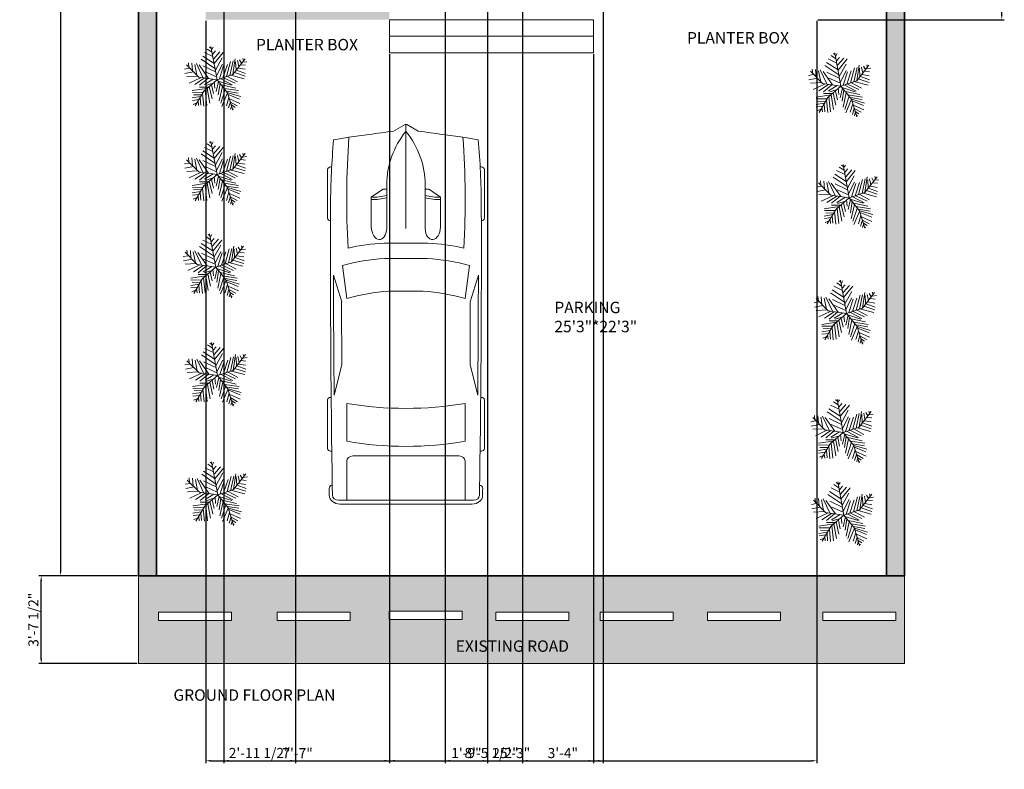
# Model space of a CAD drawing. Units: inches. Extents: x 2130 to 2621, y 981 to 1994.
# Tile 1 of 4: x 2130 to 2618, y 981 to 1353. Entities that reach past the tile are written whole.
import ezdxf

# ---------------------------------------------------------------- set-up
doc = ezdxf.new("R2010")
doc.units = ezdxf.units.IN
for name, color, linetype, lineweight in [('A-ANNO-DIMS', 2, 'Continuous', 18), ('A-ANNO-TEXT', 10, 'Continuous', 18), ('A-AREA-IDEN', 10, 'Continuous', 18), ('A-FLOR-STRS', 7, 'Continuous', 18), ('A-WALL-PATT', 140, 'Continuous', 13), ('C-PARK-VEHI', 8, 'Continuous', 18), ('C-PROP', 7, 'Continuous', 35), ('C-PROP-PATT', 140, 'Continuous', 13), ('C-ROAD-PATT', 252, 'Continuous', 13), ('ROAD', 18, 'Continuous', 18), ('TREE', 112, 'Continuous', 18)]:
    doc.layers.add(name, color=color, linetype=linetype, lineweight=lineweight)
doc.styles.get("Standard").update_dxf_attribs({"font": 'arial.ttf'})
doc.dimstyles.new('ISO-25', dxfattribs={"dimtxt": 5, "dimasz": 2.5, "dimexe": 1.25, "dimexo": 0.625, "dimtad": 1, "dimdec": 0, "dimlunit": 4, "dimtxsty": 'Standard', "dimcen": 2.5, "dimadec": 0, "dimazin": 0, "dimtfac": 1, "dimtdec": 0, "dimtmove": 0, "dimatfit": 3, "dimfxl": 1, "dimarcsym": 0})

# ---------------------------------------------------------------- blocks, each defined once
blk = doc.blocks.new('*U6')
for p, q in [((21.1, 37.41), (21.1, 36.83)), ((46.55, 38.89), (22.35, 38.89)), ((47.8, 37.39), (47.8, 37.41)), ((87.99, 31.87), (74.76, 35.92)), ((134.31, 35.6), (119.29, 31.78)), ((135.45, 37.07), (135.45, 37.41)), ((136.7, 38.89), (160.9, 38.89)), ((162.15, 37.41), (162.15, 36.77)), ((70.03, 31.54), (86.41, 29.35)), ((138.42, 29.35), (157.25, 29.35)), ((186.47, 29.35), (167.01, 29.35)), ((186.47, -33.5), (186.47, 33.5)), ((188.4, -32.76), (188.4, 32.76)), ((164.52, 26.39), (164.52, -26.39)), ((32.27, 11.63), (36.13, 17.17)), ((36.13, 17.17), (50.94, 17.17)), ((32.12, 9.51), (32.12, 11.15)), ((58.92, -10.77), (58.92, 10.77)), ((66.55, -10.53), (66.55, 10.53)), ((186.47, -10.53), (186.47, 10.53)), ((3.27, 6.13), (0.1, 0.41)), ((29.77, 9.51), (51.68, 9.51)), ((82.74, 8.5), (82.74, -8.5)), ((0, 0), (51.68, 0)), ((0.1, -0.41), (3.27, -6.13)), ((29.77, -9.51), (51.68, -9.51)), ((32.12, -9.51), (32.12, -11.15)), ((32.27, -11.63), (36.13, -17.17)), ((36.13, -17.17), (50.94, -17.17)), ((86.41, -29.35), (70.03, -31.54)), ((87.99, -31.87), (74.76, -35.92)), ((134.31, -35.6), (119.29, -31.78)), ((157.25, -29.35), (138.42, -29.35)), ((167.01, -29.35), (186.47, -29.35)), ((21.1, -37.41), (21.1, -36.83)), ((46.55, -38.89), (22.35, -38.89)), ((47.8, -37.39), (47.8, -37.41)), ((135.45, -37.07), (135.45, -37.41)), ((136.7, -38.89), (160.9, -38.89)), ((162.15, -37.41), (162.15, -36.77))]:
    blk.add_line(p, q)
for centre, major_axis, ratio, start_param, end_param in [((266.03, -27.52), (0, 313.31), 0.842304, 1.367076, 1.39176), ((41.19, -490.86), (0, 528.23), 0.842304, 0.00281, 0.075598), ((22.35, 37.41), (0, -1.48), 0.842304, 3.141593, 4.712389), ((64.48, -10555.62), (0, 10593.03), 0.842304, -0.013397, 0.002797), ((46.55, 37.41), (0, 1.48), 0.842304, -1.570796, 0), ((64.48, -10555.62), (0, -10591.55), 0.842304, 3.133765, 3.140441), ((136.7, 37.41), (0, -1.48), 0.842304, 3.141593, 4.712389), ((160.9, 37.41), (0, 1.48), 0.842304, -1.570796, 0), ((180.63, 35.84), (0, 2.22), 0.842304, -0.013017, 1.249894), ((64.48, -10556.36), (0, 10595.31), 0.842304, -0.013397, -0.013017), ((183.98, 33.5), (0, -2.96), 0.842304, 1.570796, 3.128196), ((183.98, 32.76), (0, -5.25), 0.842304, 1.570796, 3.128196), ((37.47, -593.96), (0, -623.33), 0.842304, 3.096046, 3.200911), ((135.29, 5.39), (0, 81.77), 0.842304, 1.245306, 1.50788), ((149.6, 2.8), (0, -79.58), 0.842304, 4.372215, 4.640744), ((95.79, -3666.35), (0, -3698.24), 0.842304, 3.134049, 3.144098), ((17.08, 0), (0, 147.02), 0.842304, 4.511394, 4.913384), ((35.91, 0), (0, 147.02), 0.842304, 4.511394, 4.913384), ((167.01, 26.39), (0, 2.96), 0.842304, 0, 1.570796), ((259.18, -27.52), (0, -305.3), 0.842304, 4.528606, 4.561838), ((134.4, 5.39), (0, -89.78), 0.842304, 4.449482, 4.652344), ((-204.49, 52.4), (0, -250.96), 0.842304, 1.385369, 1.434372), ((13.04, 17.01), (0, 27.42), 0.842304, 4.435146, 4.718221), ((14.2, 17.01), (0, 27.42), 0.842304, 4.435146, 4.718221), ((50.79, 13.34), (6.34, -0.36), 0.603834, -1.395552, 1.581315), ((32.75, 11.15), (0, 0.74), 0.842304, 0.879714, 1.570796), ((29.77, -46.66), (0, 56.17), 0.842304, 0, 0.590319), ((0.62, 0), (0, -0.74), 0.842304, 4.131459, 5.293319), ((29.77, 46.66), (0, 56.17), 0.842304, 2.551274, 3.141593), ((-204.49, -52.4), (0, 250.96), 0.842304, -1.434372, -1.385369), ((13.04, -17.01), (0, -27.42), 0.842304, 1.564964, 1.848039), ((14.2, -17.01), (0, -27.42), 0.842304, 1.564964, 1.848039), ((149.6, -2.8), (0, -79.58), 0.842304, -1.499151, -1.230623), ((32.75, -11.15), (0, -0.74), 0.842304, 4.712389, 5.403472), ((134.4, -5.39), (0, -89.78), 0.842304, -1.510751, -1.307889), ((135.29, -5.39), (0, -81.77), 0.842304, -1.50788, -1.245306), ((259.18, 27.52), (0, 305.3), 0.842304, 1.721348, 1.754579), ((266.03, 27.52), (0, 313.31), 0.842304, 1.749832, 1.774517), ((37.47, 593.96), (0, -623.33), 0.842304, -0.059319, 0.045547), ((167.01, -26.39), (0, -2.96), 0.842304, 4.712389, 6.283185), ((95.79, 3666.35), (0, -3698.24), 0.842304, -0.002505, 0.007544), ((183.98, -33.5), (0, 2.96), 0.842304, 3.15499, 4.712389), ((183.98, -32.76), (0, -5.25), 0.842304, 0.013397, 1.570796), ((41.19, 490.86), (0, -528.23), 0.842304, -0.075598, -0.00281), ((22.35, -37.41), (0, 1.48), 0.842304, 1.570796, 3.141593), ((64.48, 10555.62), (0, 10593.03), 0.842304, 3.138796, 3.15499), ((46.55, -37.41), (0, -1.48), 0.842304, 0, 1.570796), ((64.48, 10555.62), (0, -10591.55), 0.842304, 0.001152, 0.007828), ((136.7, -37.41), (0, -1.48), 0.842304, -1.570796, 0), ((160.9, -37.41), (0, 1.48), 0.842304, 3.141593, 4.712389), ((180.63, -35.84), (0, -2.22), 0.842304, -1.249894, 0.013017), ((64.48, 10556.36), (0, 10595.31), 0.842304, 3.15461, 3.15499)]:
    blk.add_ellipse(centre, major_axis=major_axis, ratio=ratio, start_param=start_param, end_param=end_param)
at = {"extrusion": (0, 0, -1)}
blk.add_ellipse((50.79, -13.34), major_axis=(6.34, 0.36), ratio=0.603834, start_param=-1.395552, end_param=1.581315, dxfattribs=at)
blk = doc.blocks.new('*D10')
at = {"layer": 'A-ANNO-DIMS', "color": 0, "lineweight": -2, "transparency": 16777216}
for p, q in [((2188.13, 1935.02), (2148.94, 1935.02)), ((2150.19, 1932.52), (2150.19, 1079.91)), ((2188.13, 1077.41), (2148.94, 1077.41))]:
    blk.add_line(p, q, dxfattribs=at)
at = {"layer": 'A-ANNO-DIMS', "color": 0, "transparency": 16777216}
for points in [[(2149.77, 1932.52), (2150.61, 1932.52), (2150.19, 1935.02)], [(2149.77, 1079.91), (2150.61, 1079.91), (2150.19, 1077.41)]]:
    blk.add_solid(points, dxfattribs=at)
at = {"layer": 'Defpoints', "color": 0, "transparency": 16777216}
for p in [(2188.76, 1935.02), (2150.19, 1077.41), (2188.76, 1077.41)]:
    blk.add_point(p, dxfattribs=at)
at = {"layer": 'A-ANNO-DIMS', "color": 0, "transparency": 16777216, "insert": (2147.01, 1506.21), "char_height": 5, "attachment_point": 5, "rotation": 90}
blk.add_mtext('71\'-6"', dxfattribs=at)
blk = doc.blocks.new('*U8')
for p, q in [((-8.737, 47.138), (-17.069, 52.711)), ((-10.186, 53.64), (-13.084, 55.962)), ((0, 0), (-10.5, 57)), ((-9.099, 51.782), (-6.563, 55.962)), ((-3.665, 19.273), (-27.574, 35.527)), ((-5.114, 28.097), (-24.676, 40.636)), ((-7.288, 39.707), (-21.778, 46.673)), ((-7.65, 43.423), (-2.578, 49.46)), ((-5.839, 35.992), (4.667, 48.067)), ((-5.114, 27.632), (10.463, 46.673)), ((-2.941, 16.486), (8.652, 37.85)), ((27, 9), (48, 36)), ((27.127, 9.056), (31.112, 35.992)), ((38.719, 34.134), (41.979, 28.561)), ((44.153, 36.456), (45.239, 32.741)), ((-47.498, 19.737), (-55.83, 18.344)), ((-31.5, 4.5), (-52.5, 25.5)), ((-48.585, 21.131), (-49.309, 29.026)), ((-43.513, 28.561), (-42.427, 15.558)), ((-38.442, 26.239), (-34.819, 7.663)), ((-35.544, 28.097), (-24.314, 3.947)), ((-14.533, 2.09), (-30.834, 25.31)), ((-24.314, 23.917), (-2.941, 13.7)), ((-1.129, 6.734), (9.014, 26.704)), ((3.942, 1.625), (11.187, 24.381)), ((10.101, 3.483), (17.708, 26.239)), ((16.259, 5.805), (23.142, 31.348)), ((22.055, 7.198), (27.489, 32.277)), ((31.836, 30.883), (32.561, 16.486)), ((35.096, 32.741), (37.27, 22.524)), ((36.183, 19.737), (48.137, 17.88)), ((40.53, 25.775), (48.862, 24.846)), ((43.791, 29.954), (51.036, 30.883)), ((-40.615, 13.7), (-55.105, 10.913)), ((-33.37, 6.269), (-52.207, 5.34)), ((-28.299, 3.483), (-47.86, -5.805)), ((-21.416, 3.018), (-38.079, -8.128)), ((0, 0), (-31.5, 4.5)), ((-15.982, 2.09), (-30.11, -9.521)), ((0, 0), (-22.5, -19.5)), ((-6.563, 1.161), (-21.416, -8.128)), ((-20.691, 13.7), (-1.129, 4.876)), ((0, 0), (27, 9)), ((0, 0), (18, -22.5)), ((6.478, 1.625), (26.04, -8.592)), ((11.187, 3.483), (30.749, -5.805)), ((18.07, 5.805), (35.096, -3.483)), ((24.229, 7.663), (46.688, 1.625)), ((29.662, 12.307), (48.137, 6.269)), ((33.285, 16.486), (48.862, 10.913)), ((-17.431, -15.094), (-42.789, -18.809)), ((-15.257, -12.772), (-30.11, -12.772)), ((-6.563, -5.805), (-19.967, -9.985)), ((-17.069, -15.094), (-12.721, -40.172)), ((-13.446, -11.378), (-8.737, -32.741)), ((-9.461, -8.592), (-6.201, -23.453)), ((-4.752, -3.483), (-3.665, -14.629)), ((2.493, -3.019), (-1.491, -20.202)), ((1.769, -2.555), (24.229, -9.521)), ((5.029, -6.27), (2.131, -25.775)), ((9.014, -11.378), (3.58, -35.992)), ((7.565, -9.056), (32.198, -14.629)), ((12.274, -15.094), (36.907, -18.809)), ((-28.299, -29.026), (-42.789, -31.348)), ((-24.314, -21.596), (-42.427, -22.06)), ((-26.849, -26.24), (-40.253, -25.775)), ((-22.5, -19.5), (-37.5, -45)), ((-29.023, -30.884), (-27.936, -43.887)), ((-25.038, -23.918), (-22.865, -45.281)), ((-20.691, -18.345), (-17.793, -44.352)), ((14.085, -16.951), (6.478, -40.172)), ((18.07, -22.524), (8.289, -45.745)), ((20.244, -30.419), (15.897, -44.816)), ((16.259, -19.738), (36.183, -22.989)), ((18, -22.5), (27, -52.5)), ((18.433, -22.524), (40.53, -29.026)), ((19.157, -25.311), (38.719, -33.206)), ((21.331, -32.741), (39.081, -40.636)), ((-30.834, -34.135), (-42.427, -35.528)), ((-34.457, -39.708), (-40.978, -42.494)), ((-32.646, -36.921), (-31.921, -44.352)), ((22.78, -37.85), (19.519, -48.532)), ((22.78, -38.314), (34.372, -44.816)), ((24.591, -45.745), (23.142, -50.854)), ((24.591, -43.423), (30.749, -47.603)), ((26.764, -49.925), (28.213, -50.854))]:
    blk.add_line(p, q)
blk = doc.blocks.new('*D23')
at = {"layer": 'A-ANNO-DIMS', "color": 0, "lineweight": -2, "transparency": 16777216}
for p, q in [((2222.16, 1352.79), (2222.16, 984.42)), ((2525.16, 1352.79), (2525.16, 984.42)), ((2224.66, 985.67), (2522.66, 985.67))]:
    blk.add_line(p, q, dxfattribs=at)
at = {"layer": 'A-ANNO-DIMS', "color": 0, "transparency": 16777216}
for points in [[(2224.66, 986.08), (2224.66, 985.25), (2222.16, 985.67)], [(2522.66, 986.08), (2522.66, 985.25), (2525.16, 985.67)]]:
    blk.add_solid(points, dxfattribs=at)
at = {"layer": 'Defpoints', "color": 0, "transparency": 16777216}
for p in [(2222.16, 1353.41), (2525.16, 1353.41), (2525.16, 985.67)]:
    blk.add_point(p, dxfattribs=at)
at = {"layer": 'A-ANNO-DIMS', "color": 0, "transparency": 16777216, "insert": (2373.66, 988.85), "char_height": 5, "attachment_point": 5}
blk.add_mtext('25\'-3"', dxfattribs=at)
blk = doc.blocks.new('*D24')
at = {"layer": 'A-ANNO-DIMS', "color": 0, "lineweight": -2, "transparency": 16777216}
for p, q in [((2525.79, 1890.41), (2618.19, 1890.41)), ((2616.94, 1355.91), (2616.94, 1887.91)), ((2525.79, 1353.41), (2618.19, 1353.41))]:
    blk.add_line(p, q, dxfattribs=at)
at = {"layer": 'A-ANNO-DIMS', "color": 0, "transparency": 16777216}
for points in [[(2616.52, 1887.91), (2617.35, 1887.91), (2616.94, 1890.41)], [(2616.52, 1355.91), (2617.35, 1355.91), (2616.94, 1353.41)]]:
    blk.add_solid(points, dxfattribs=at)
at = {"layer": 'Defpoints', "color": 0, "transparency": 16777216}
for p in [(2525.16, 1890.41), (2616.94, 1890.41), (2525.16, 1353.41)]:
    blk.add_point(p, dxfattribs=at)
at = {"layer": 'A-ANNO-DIMS', "color": 0, "transparency": 16777216, "insert": (2613.76, 1621.91), "char_height": 5, "attachment_point": 5, "rotation": 90}
blk.add_mtext('44\'-9"', dxfattribs=at)
blk = doc.blocks.new('*D27')
at = {"layer": 'A-ANNO-DIMS', "color": 0, "lineweight": -2, "transparency": 16777216}
for p, q in [((2188.13, 1077.41), (2139.33, 1077.41)), ((2140.58, 1036.35), (2140.58, 1074.91)), ((2188.13, 1033.85), (2139.33, 1033.85))]:
    blk.add_line(p, q, dxfattribs=at)
at = {"layer": 'A-ANNO-DIMS', "color": 0, "transparency": 16777216}
for points in [[(2140.16, 1074.91), (2140.99, 1074.91), (2140.58, 1077.41)], [(2140.16, 1036.35), (2140.99, 1036.35), (2140.58, 1033.85)]]:
    blk.add_solid(points, dxfattribs=at)
at = {"layer": 'Defpoints', "color": 0, "transparency": 16777216}
for p in [(2140.58, 1077.41), (2188.76, 1077.41), (2188.76, 1033.85)]:
    blk.add_point(p, dxfattribs=at)
at = {"layer": 'A-ANNO-DIMS', "color": 0, "transparency": 16777216, "insert": (2137.36, 1055.63), "char_height": 5, "attachment_point": 5, "rotation": 90}
blk.add_mtext('3\'-7 1/2"', dxfattribs=at)
blk = doc.blocks.new('*D30')
at = {"layer": 'A-ANNO-DIMS', "color": 0, "lineweight": -2, "transparency": 16777216}
for p, q in [((2313.28, 1336.32), (2313.28, 984.42)), ((2414.54, 1336.32), (2414.54, 984.42)), ((2315.78, 985.67), (2412.04, 985.67))]:
    blk.add_line(p, q, dxfattribs=at)
at = {"layer": 'A-ANNO-DIMS', "color": 0, "transparency": 16777216}
for points in [[(2315.78, 986.08), (2315.78, 985.25), (2313.28, 985.67)], [(2412.04, 986.08), (2412.04, 985.25), (2414.54, 985.67)]]:
    blk.add_solid(points, dxfattribs=at)
at = {"layer": 'Defpoints', "color": 0, "transparency": 16777216}
for p in [(2313.28, 1336.95), (2414.54, 1336.95), (2414.54, 985.67)]:
    blk.add_point(p, dxfattribs=at)
at = {"layer": 'A-ANNO-DIMS', "color": 0, "transparency": 16777216, "insert": (2363.91, 988.88), "char_height": 5, "attachment_point": 5}
blk.add_mtext('8\'-5 1/2"', dxfattribs=at)
blk = doc.blocks.new('*D31')
at = {"layer": 'A-ANNO-DIMS', "color": 0, "lineweight": -2, "transparency": 16777216}
for p, q in [((2222.16, 1352.79), (2222.16, 984.42)), ((2313.28, 1336.32), (2313.28, 984.42)), ((2224.66, 985.67), (2310.78, 985.67))]:
    blk.add_line(p, q, dxfattribs=at)
at = {"layer": 'A-ANNO-DIMS', "color": 0, "transparency": 16777216}
for points in [[(2224.66, 986.08), (2224.66, 985.25), (2222.16, 985.67)], [(2310.78, 986.08), (2310.78, 985.25), (2313.28, 985.67)]]:
    blk.add_solid(points, dxfattribs=at)
at = {"layer": 'Defpoints', "color": 0, "transparency": 16777216}
for p in [(2222.16, 1353.41), (2313.28, 1336.95), (2313.28, 985.67)]:
    blk.add_point(p, dxfattribs=at)
at = {"layer": 'A-ANNO-DIMS', "color": 0, "transparency": 16777216, "insert": (2267.72, 988.79), "char_height": 5, "attachment_point": 5}
blk.add_mtext('7\'-7"', dxfattribs=at)
blk = doc.blocks.new('*D33')
at = {"layer": 'A-ANNO-DIMS', "color": 0, "lineweight": -2, "transparency": 16777216}
for p, q in [((2231.16, 1510.29), (2231.16, 984.42)), ((2266.66, 1510.29), (2266.66, 984.42)), ((2233.66, 985.67), (2264.16, 985.67))]:
    blk.add_line(p, q, dxfattribs=at)
at = {"layer": 'A-ANNO-DIMS', "color": 0, "transparency": 16777216}
for points in [[(2233.66, 986.08), (2233.66, 985.25), (2231.16, 985.67)], [(2264.16, 986.08), (2264.16, 985.25), (2266.66, 985.67)]]:
    blk.add_solid(points, dxfattribs=at)
at = {"layer": 'Defpoints', "color": 0, "transparency": 16777216}
for p in [(2231.16, 1510.91), (2266.66, 1510.91), (2266.66, 985.67)]:
    blk.add_point(p, dxfattribs=at)
at = {"layer": 'A-ANNO-DIMS', "color": 0, "transparency": 16777216, "insert": (2248.91, 988.88), "char_height": 5, "attachment_point": 5}
blk.add_mtext('2\'-11 1/2"', dxfattribs=at)
blk = doc.blocks.new('*D36')
at = {"layer": 'A-ANNO-DIMS', "color": 0, "lineweight": -2, "transparency": 16777216}
for p, q in [((2379.27, 1730.79), (2379.27, 984.42)), ((2419.27, 1730.79), (2419.27, 984.42)), ((2381.77, 985.67), (2416.77, 985.67))]:
    blk.add_line(p, q, dxfattribs=at)
at = {"layer": 'A-ANNO-DIMS', "color": 0, "transparency": 16777216}
for points in [[(2381.77, 986.08), (2381.77, 985.25), (2379.27, 985.67)], [(2416.77, 986.08), (2416.77, 985.25), (2419.27, 985.67)]]:
    blk.add_solid(points, dxfattribs=at)
at = {"layer": 'Defpoints', "color": 0, "transparency": 16777216}
for p in [(2379.27, 1731.41), (2419.27, 1731.41), (2419.27, 985.67)]:
    blk.add_point(p, dxfattribs=at)
at = {"layer": 'A-ANNO-DIMS', "color": 0, "transparency": 16777216, "insert": (2399.27, 988.85), "char_height": 5, "attachment_point": 5}
blk.add_mtext('3\'-4"', dxfattribs=at)
blk = doc.blocks.new('*D45')
at = {"layer": 'A-ANNO-DIMS', "color": 0, "lineweight": -2, "transparency": 16777216}
for p, q in [((2340.91, 1828.29), (2340.91, 984.42)), ((2361.98, 1828.29), (2361.98, 984.42)), ((2343.41, 985.67), (2359.48, 985.67))]:
    blk.add_line(p, q, dxfattribs=at)
at = {"layer": 'A-ANNO-DIMS', "color": 0, "transparency": 16777216}
for points in [[(2343.41, 986.08), (2343.41, 985.25), (2340.91, 985.67)], [(2359.48, 986.08), (2359.48, 985.25), (2361.98, 985.67)]]:
    blk.add_solid(points, dxfattribs=at)
at = {"layer": 'Defpoints', "color": 0, "transparency": 16777216}
for p in [(2340.91, 1828.91), (2361.98, 1828.91), (2361.98, 985.67)]:
    blk.add_point(p, dxfattribs=at)
at = {"layer": 'A-ANNO-DIMS', "color": 0, "transparency": 16777216, "insert": (2351.44, 988.84), "char_height": 5, "attachment_point": 5}
blk.add_mtext('1\'-9"', dxfattribs=at)

msp = doc.modelspace()

# ---------------------------------------------------------------- hatches: boundary and pattern name
at = {"layer": 'A-WALL-PATT'}
h = msp.add_hatch(color=256, dxfattribs=at)
h.dxf.hatch_style = 1
h.paths.add_polyline_path([(2231.16, 1595.8), (2222.16, 1595.8), (2222.16, 1571.6), (2225.81, 1571.6), (2231.16, 1571.6)])
h.paths.add_polyline_path([(2313.28, 1362.41), (2237.26, 1362.41), (2231.16, 1362.41), (2231.16, 1404.41), (2231.16, 1474.85), (2231.16, 1547.86, -0.05547), (2225.81, 1547.27), (2222.16, 1547.27), (2222.16, 1425.41), (2222.16, 1353.41), (2313.28, 1353.41)])
h.paths.add_polyline_path([(2393.01, 1195.09), (2434.46, 1195.09), (2434.46, 1216.28), (2393.01, 1216.28)], flags=9)
h.paths.add_polyline_path([(2245.08, 1335), (2303.47, 1335), (2303.47, 1346.7), (2245.08, 1346.7)], flags=9)
h.paths.add_polyline_path([(2458.81, 1338.38), (2517.21, 1338.38), (2517.21, 1350.09), (2458.81, 1350.09)], flags=9)
h.paths.add_polyline_path([(2232.7, 1530.42), (2263.31, 1530.42), (2263.31, 1551.62), (2232.7, 1551.62)], flags=9)
h.paths.add_polyline_path([(2332.94, 1458.61), (2399.05, 1458.61), (2399.05, 1489.37), (2332.94, 1489.37)], flags=9)
h.paths.add_polyline_path([(2475.66, 1607.66), (2507.9, 1607.66), (2507.9, 1628.85), (2475.66, 1628.85)], flags=9)
h.paths.add_polyline_path([(2486.7, 1688.97), (2517.32, 1688.97), (2517.32, 1710.17), (2486.7, 1710.17)], flags=9)
h.paths.add_polyline_path([(2333.88, 1649.81), (2375.07, 1649.81), (2375.07, 1671), (2333.88, 1671)], flags=9)
h.paths.add_polyline_path([(2441.42, 1774.34), (2500.24, 1774.34), (2500.24, 1795.53), (2441.42, 1795.53)], flags=9)
h.paths.add_polyline_path([(2332.74, 1857.16), (2363.5, 1857.16), (2363.5, 1878.35), (2332.74, 1878.35)], flags=9)
h.paths.add_polyline_path([(2244.84, 1853.21), (2275.6, 1853.21), (2275.6, 1874.4), (2244.84, 1874.4)], flags=9)
at = {"layer": 'C-PROP-PATT'}
h = msp.add_hatch(color=256, dxfattribs=at)
h.dxf.hatch_style = 1
h.paths.add_polyline_path([(2559.76, 1935.02), (2197.76, 1935.02), (2197.76, 1926.02), (2559.76, 1926.02)])
h.paths.add_polyline_path([(2197.76, 1935.02), (2188.76, 1935.02), (2188.76, 1077.41), (2197.76, 1077.41)])
h.paths.add_polyline_path([(2568.76, 1926.02), (2559.76, 1926.02), (2559.76, 1077.41), (2568.76, 1077.41)])
h.paths.add_polyline_path([(2568.76, 1935.02), (2559.76, 1935.02), (2559.76, 1926.02), (2568.76, 1926.02)])
at = {"layer": 'C-ROAD-PATT'}
h = msp.add_hatch(color=256, dxfattribs=at)
h.dxf.hatch_style = 1
h.paths.add_polyline_path([(2568.76, 1077.41), (2559.76, 1077.41), (2188.76, 1077.41), (2188.76, 1033.85), (2568.76, 1033.85)])
h.paths.add_polyline_path([(2349.31, 1059.97), (2349.31, 1055.82), (2313.18, 1055.82), (2313.18, 1059.97)], flags=16)
h.paths.add_polyline_path([(2366.11, 1059.44), (2402.25, 1059.44), (2402.25, 1055.28), (2366.11, 1055.28)], flags=16)
h.paths.add_polyline_path([(2417.78, 1059.44), (2453.92, 1059.44), (2453.92, 1055.28), (2417.78, 1055.28)], flags=16)
h.paths.add_polyline_path([(2293.74, 1059.44), (2293.74, 1055.28), (2257.61, 1055.28), (2257.61, 1059.44)], flags=16)
h.paths.add_polyline_path([(2471.02, 1059.44), (2507.15, 1059.44), (2507.15, 1055.28), (2471.02, 1055.28)], flags=16)
h.paths.add_polyline_path([(2234.9, 1059.44), (2234.9, 1055.28), (2198.77, 1055.28), (2198.77, 1059.44)], flags=16)
h.paths.add_polyline_path([(2528.27, 1059.44), (2564.4, 1059.44), (2564.4, 1055.28), (2528.27, 1055.28)], flags=16)
h.paths.add_polyline_path([(2344.06, 1036.51), (2409.07, 1036.51), (2409.07, 1048.22), (2344.06, 1048.22)], flags=24)

# ---------------------------------------------------------------- linework, layer by layer
at = {"layer": 'A-FLOR-STRS'}
for points in [[(2313.28, 1353.41), (2414.44, 1353.41), (2414.44, 1345.18), (2313.28, 1345.18)], [(2313.28, 1345.18), (2414.54, 1345.18), (2414.54, 1336.95), (2313.28, 1336.95)]]:
    msp.add_lwpolyline(points, close=True, dxfattribs=at)
at = {"layer": 'C-PROP'}
for p, q in [((2188.76, 1935.02), (2188.76, 1077.41)), ((2568.76, 1935.02), (2568.76, 1077.41)), ((2197.76, 1926.02), (2197.76, 1086.41)), ((2559.76, 1926.02), (2559.76, 1086.41)), ((2197.76, 1086.41), (2197.76, 1077.41)), ((2559.76, 1086.41), (2559.76, 1077.41)), ((2568.76, 1077.41), (2188.76, 1077.41))]:
    msp.add_line(p, q, dxfattribs=at)
for points in [[(2188.76, 1935.02), (2197.76, 1935.02), (2197.76, 1077.41), (2188.76, 1077.41)], [(2559.76, 1077.41), (2568.76, 1077.41), (2568.76, 1935.02), (2559.76, 1935.02)]]:
    msp.add_lwpolyline(points, close=True, dxfattribs=at)
at = {"layer": 'ROAD'}
for p, q in [((2188.76, 1077.41), (2188.76, 1033.85)), ((2568.76, 1033.85), (2568.76, 1077.41)), ((2188.76, 1033.85), (2568.76, 1033.85))]:
    msp.add_line(p, q, dxfattribs=at)
for points in [[(2313.18, 1059.97), (2349.31, 1059.97), (2349.31, 1055.82), (2313.18, 1055.82)], [(2198.77, 1059.44), (2234.9, 1059.44), (2234.9, 1055.28), (2198.77, 1055.28)], [(2257.61, 1059.44), (2293.74, 1059.44), (2293.74, 1055.28), (2257.61, 1055.28)], [(2366.11, 1059.44), (2402.25, 1059.44), (2402.25, 1055.28), (2366.11, 1055.28)], [(2417.78, 1059.44), (2453.92, 1059.44), (2453.92, 1055.28), (2417.78, 1055.28)], [(2471.02, 1059.44), (2507.15, 1059.44), (2507.15, 1055.28), (2471.02, 1055.28)], [(2528.27, 1059.44), (2564.4, 1059.44), (2564.4, 1055.28), (2528.27, 1055.28)]]:
    msp.add_lwpolyline(points, close=True, dxfattribs=at)

# ---------------------------------------------------------------- block references
at = {"layer": 'C-PARK-VEHI', "rotation": 270}
msp.add_blockref('*U6', (2321.45, 1301.43), dxfattribs=at)
at = {"layer": 'TREE', "xscale": 0.2888583255647464, "yscale": 0.2888583255647464, "zscale": 0.2888583255647464}
for p in [(2227.8, 1323.62), (2537.2, 1320.43), (2227.8, 1276.57), (2541.25, 1265.04), (2227.1, 1230.6), (2540, 1207.62), (2228.01, 1176.8), (2538.33, 1148.63), (2228.14, 1117.6), (2538.65, 1107.56)]:
    msp.add_blockref('*U8', p, dxfattribs=at)

# ---------------------------------------------------------------- texts
at = {"layer": 'A-ANNO-TEXT', "char_height": 5.6797, "attachment_point": 1}
for s, width, insert in [('PLANTER BOX', 57.6358, (2247.11, 1343.88)), ('PLANTER BOX', 57.6358, (2460.84, 1347.27)), ('EXISTING ROAD', 79.6446, (2346.11, 1045.4)), ('GROUND FLOOR PLAN', 98.7305, (2206.15, 1021.11))]:
    msp.add_mtext_dynamic_manual_height_columns(s, width=width, gutter_width=28.4, heights=[0], dxfattribs=dict(at, insert=insert))
at = {"layer": 'A-AREA-IDEN', "insert": (2395.04, 1213.46), "char_height": 5.6797, "attachment_point": 1}
msp.add_mtext_dynamic_manual_height_columns('PARKING\\P25\'3"*22\'3"', width=57.6358, gutter_width=28.4, heights=[0], dxfattribs=at)

# ---------------------------------------------------------------- dimensions: what is measured, and where the dimension line sits
at = {"layer": 'A-ANNO-DIMS'}
for base, p1, p2, override, picture, middle in [((2150.19, 1077.41), (2188.76, 1935.02), (2188.76, 1077.41), {"dimclrd": 0, "dimclre": 0, "dimclrt": 0}, '*D10', (2147.01, 1506.21)), ((2616.94, 1890.41), (2525.16, 1353.41), (2525.16, 1890.41), {"dimdec": 1, "dimlfac": 1, "dimrnd": 0, "dimzin": 1, "dimdsep": 46, "dimlunit": 4, "dimfrac": 2}, '*D24', (2613.76, 1621.91)), ((2140.58, 1077.41), (2188.76, 1033.85), (2188.76, 1077.41), {"dimdec": 1, "dimlfac": 1, "dimrnd": 0, "dimzin": 1, "dimdsep": 46, "dimlunit": 4, "dimfrac": 2}, '*D27', (2137.36, 1055.63))]:
    dim = msp.add_linear_dim(base=base, p1=p1, p2=p2, angle=90, dimstyle='ISO-25', override=override, dxfattribs=at)
    dim.commit()
    dim.dimension.update_dxf_attribs({"geometry": picture, "text_midpoint": middle})
for base, p1, p2, picture, middle in [((2361.98, 985.67), (2340.91, 1828.91), (2361.98, 1828.91), '*D45', (2351.44, 988.84)), ((2419.27, 985.67), (2379.27, 1731.41), (2419.27, 1731.41), '*D36', (2399.27, 988.85)), ((2266.66, 985.67), (2231.16, 1510.91), (2266.66, 1510.91), '*D33', (2248.91, 988.88)), ((2525.16, 985.67), (2222.16, 1353.41), (2525.16, 1353.41), '*D23', (2373.66, 988.85)), ((2313.28, 985.67), (2222.16, 1353.41), (2313.28, 1336.95), '*D31', (2267.72, 988.79)), ((2414.54, 985.67), (2313.28, 1336.95), (2414.54, 1336.95), '*D30', (2363.91, 988.88))]:
    dim = msp.add_linear_dim(base=base, p1=p1, p2=p2, dimstyle='ISO-25', override={"dimdec": 1, "dimlfac": 1, "dimrnd": 0, "dimzin": 1, "dimdsep": 46, "dimlunit": 4, "dimfrac": 2}, dxfattribs=at)
    dim.commit()
    dim.dimension.update_dxf_attribs({"geometry": picture, "text_midpoint": middle})

doc.saveas('drawing.dxf')
